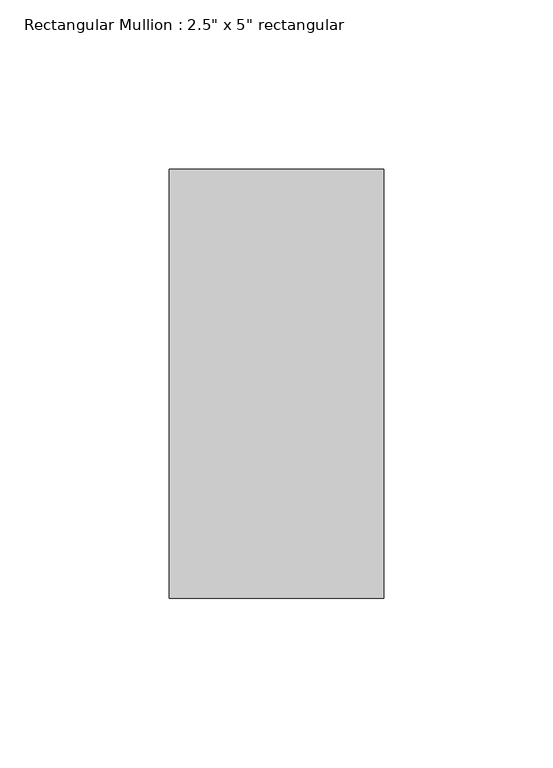
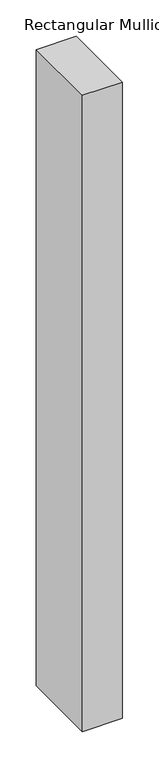
"""IFC4 building model written with IfcOpenShell, lengths in millimetres: member geometry."""

from ifc_helpers import new_model, si_unit, frame, origin, place, context, project, spatial, polyline, outline, extrude, source, transform, mapped, element, save


def member_693dcaa1(model_context):
    return source(origin(), model_context, "Body", "SweptSolid", [
        extrude(outline(polyline([(0.0, 63.5), (0.0, -63.5), (-63.5, -63.5), (-63.5, 63.5), (0.0, 63.5)])), frame((0.0, 0.0, -1068.9166668), z_axis=(0.0, 0.0, 1.0), x_axis=(1.0, 0.0, 0.0)), (0.0, 0.0, 1.0), 1068.9166668),
    ])


if __name__ == "__main__":
    model = new_model("IFC4")
    model_context = context("Model", 3, world=origin())
    ifc_project = project(units=[si_unit("LENGTHUNIT", "METRE", prefix="MILLI")], contexts=[model_context])
    site = spatial("IfcSite", under=ifc_project)
    building = spatial("IfcBuilding", under=site)
    placement = place(None, origin())
    member_shape = member_693dcaa1(model_context)
    element("IfcMember", 1, ObjectType="Rectangular Mullion : 2.5\" x 5\" rectangular", at=placement, inside=building, context=model_context, shape_type="MappedRepresentation", body=[
        mapped(member_shape, transform((0.0, 0.0, 0.0), x_axis=(1.0, 0.0, 0.0), y_axis=(0.0, 1.0, 0.0), z_axis=(0.0, 0.0, 1.0))),
    ])
    save(model, "model.ifc")

# Revit data of these elements
# Type "Rectangular Mullion : 2.5\" x 5\" rectangular"
#   built-in parameter 1007304 = 0.416667 (stored number, unit not read)
#   built-in parameter 1007301 = 0.104167 (stored number, unit not read)
#   built-in parameter 1007300 = 0.104167 (stored number, unit not read)
# Element 1 (IfcMember, "Rectangular Mullion : 2.5\" x 5\" rectangular")
#   Materials on its faces: "metal black"
# Materials
#   "metal black": class "Generic", colour RGB 120 120 120, transparency 0, Cost = 0
